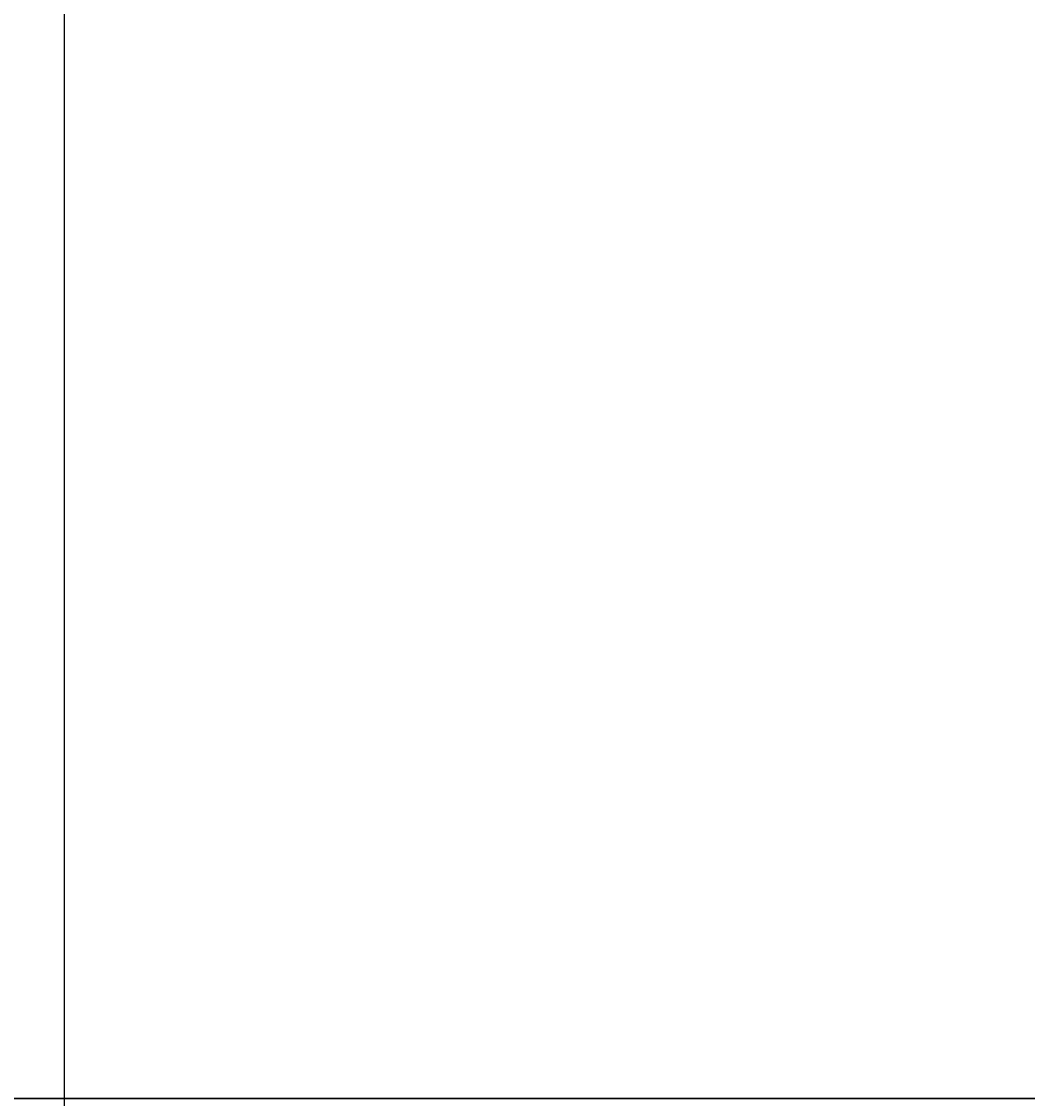
# Model space of a CAD drawing. Units: inches. Extents: x 1998 to 2588, y 1139 to 1977.
# Tile 94 of 134: x 2344 to 2397, y 1523 to 1580. Entities that reach past the tile are written whole.
import ezdxf

# ---------------------------------------------------------------- set-up
doc = ezdxf.new("R2010")
doc.units = ezdxf.units.IN
doc.layers.add('A-ANNO-DIMS', color=2, linetype='Continuous', lineweight=18)
doc.styles.get("Standard").update_dxf_attribs({"font": 'arial.ttf'})
doc.dimstyles.get("Standard").update_dxf_attribs({"dimtxt": 0.18, "dimasz": 0.18, "dimexe": 0.18, "dimexo": 0.0625, "dimgap": 0.09, "dimtad": 0, "dimtih": 1, "dimtoh": 1, "dimdec": 4, "dimzin": 0, "dimdsep": 46, "dimtxsty": 'Standard', "dimcen": 0.09, "dimadec": 0, "dimazin": 0, "dimtfac": 1, "dimtdec": 4, "dimtofl": 0, "dimtmove": 0, "dimatfit": 3, "dimfxl": 1, "dimtolj": 1, "dimtzin": 0, "dimarcsym": 0})

# ---------------------------------------------------------------- blocks, each defined once
blk = doc.blocks.new('*D34')
at = {"layer": 'A-ANNO-DIMS', "color": 0, "lineweight": -2, "transparency": 16777216}
for p, q in [((2407.91, 1594.732), (1997.843, 1594.732)), ((1998.023, 1594.552), (1998.023, 1558.913)), ((1998.023, 1522.912), (1998.023, 1558.552)), ((2407.91, 1522.732), (1997.843, 1522.732))]:
    blk.add_line(p, q, dxfattribs=at)
at = {"layer": 'A-ANNO-DIMS', "color": 0, "transparency": 16777216}
for points in [[(1997.993, 1594.552), (1998.053, 1594.552), (1998.023, 1594.732)], [(1997.993, 1522.912), (1998.053, 1522.912), (1998.023, 1522.732)]]:
    blk.add_solid(points, dxfattribs=at)
at = {"layer": 'Defpoints', "color": 0, "transparency": 16777216}
for p in [(1998.023, 1594.732), (2407.973, 1594.732), (2407.973, 1522.732)]:
    blk.add_point(p, dxfattribs=at)
at = {"layer": 'A-ANNO-DIMS', "color": 0, "transparency": 16777216, "insert": (1998.023, 1558.732), "char_height": 0.18, "attachment_point": 5}
blk.add_mtext('\\A1;72', dxfattribs=at)
blk = doc.blocks.new('*D42')
at = {"layer": 'A-ANNO-DIMS', "color": 0, "lineweight": -2, "transparency": 16777216}
for p, q in [((2287.535, 1588.732), (2588.309, 1588.732)), ((2588.129, 1588.552), (2588.129, 1555.914)), ((2588.129, 1522.912), (2588.129, 1555.55)), ((2287.535, 1522.732), (2588.309, 1522.732))]:
    blk.add_line(p, q, dxfattribs=at)
at = {"layer": 'A-ANNO-DIMS', "color": 0, "transparency": 16777216}
for points in [[(2588.099, 1588.552), (2588.159, 1588.552), (2588.129, 1588.732)], [(2588.099, 1522.912), (2588.159, 1522.912), (2588.129, 1522.732)]]:
    blk.add_solid(points, dxfattribs=at)
at = {"layer": 'Defpoints', "color": 0, "transparency": 16777216}
for p in [(2287.473, 1588.732), (2588.129, 1588.732), (2287.473, 1522.732)]:
    blk.add_point(p, dxfattribs=at)
at = {"layer": 'A-ANNO-DIMS', "color": 0, "transparency": 16777216, "insert": (2588.129, 1555.732), "char_height": 0.18, "attachment_point": 5}
blk.add_mtext('\\A1;66', dxfattribs=at)
blk = doc.blocks.new('*D43')
at = {"layer": 'A-ANNO-DIMS', "color": 0, "lineweight": -2, "transparency": 16777216}
for p, q in [((2407.973, 1594.67), (2407.973, 1138.602)), ((2345.973, 1588.67), (2345.973, 1138.602)), ((2346.153, 1138.782), (2376.754, 1138.782)), ((2407.793, 1138.782), (2377.191, 1138.782))]:
    blk.add_line(p, q, dxfattribs=at)
at = {"layer": 'A-ANNO-DIMS', "color": 0, "transparency": 16777216}
for points in [[(2346.153, 1138.812), (2346.153, 1138.752), (2345.973, 1138.782)], [(2407.793, 1138.812), (2407.793, 1138.752), (2407.973, 1138.782)]]:
    blk.add_solid(points, dxfattribs=at)
at = {"layer": 'Defpoints', "color": 0, "transparency": 16777216}
for p in [(2407.973, 1594.732), (2345.973, 1588.732), (2407.973, 1138.782)]:
    blk.add_point(p, dxfattribs=at)
at = {"layer": 'A-ANNO-DIMS', "color": 0, "transparency": 16777216, "insert": (2376.973, 1138.782), "char_height": 0.18, "attachment_point": 5}
blk.add_mtext('\\A1;62', dxfattribs=at)

msp = doc.modelspace()

# ---------------------------------------------------------------- dimensions: what is measured, and where the dimension line sits
at = {"layer": 'A-ANNO-DIMS'}
for base, p1, p2, picture, middle in [((1998.0229, 1594.7324), (2407.9729, 1522.7324), (2407.9729, 1594.7324), '*D34', (1998.0229, 1558.7324)), ((2588.1286, 1588.7324), (2287.4729, 1522.7324), (2287.4729, 1588.7324), '*D42', (2588.1286, 1555.7324))]:
    dim = msp.add_linear_dim(base=base, p1=p1, p2=p2, angle=90, dimstyle='Standard', override={"dimdec": 0, "dimlfac": 1, "dimrnd": 0, "dimzin": 0, "dimdsep": 46, "dimlunit": 2}, dxfattribs=at)
    dim.commit()
    dim.dimension.update_dxf_attribs({"geometry": picture, "text_midpoint": middle})
dim = msp.add_linear_dim(base=(2407.9729, 1138.7824), p1=(2345.9729, 1588.7324), p2=(2407.9729, 1594.7324), dimstyle='Standard', override={"dimdec": 0, "dimlfac": 1, "dimrnd": 0, "dimzin": 0, "dimdsep": 46, "dimlunit": 2}, dxfattribs=at)
dim.commit()
dim.dimension.update_dxf_attribs({"geometry": '*D43', "text_midpoint": (2376.9729, 1138.7824)})

doc.saveas('drawing.dxf')
